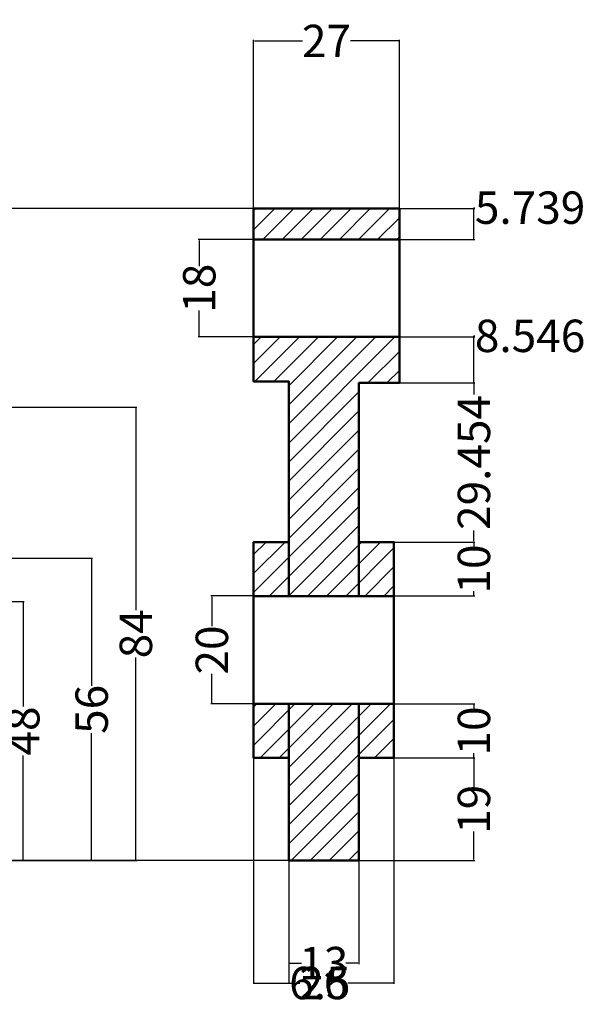
# Model space of a CAD drawing. Units: millimetres. Extents: x -1 to 307, y 9 to 193.
# Tile 2 of 2: x 203 to 307, y 11 to 193. Entities that reach past the tile are written whole.
import ezdxf

# ---------------------------------------------------------------- set-up
doc = ezdxf.new("R2010")
doc.units = ezdxf.units.MM
doc.header["$MEASUREMENT"] = 0
for name, color, linetype, lineweight in [('M-DIMS', 2, 'Continuous', 25), ('M-HATC', 8, 'Continuous', 18), ('M-OUTL', 7, 'Continuous', 50)]:
    doc.layers.add(name, color=color, linetype=linetype, lineweight=lineweight)
doc.styles.get("Standard").update_dxf_attribs({"font": 'arial.ttf'})
doc.dimstyles.get("Standard").update_dxf_attribs({"dimtxt": 6, "dimasz": 0.18, "dimexe": 0.18, "dimexo": 0.0625, "dimgap": 0.09, "dimtad": 0, "dimtoh": 1, "dimdec": 0, "dimzin": 0, "dimdsep": 46, "dimtxsty": 'Standard', "dimcen": 0.09, "dimadec": 0, "dimazin": 0, "dimtfac": 1, "dimtdec": 0, "dimtofl": 0, "dimtmove": 0, "dimatfit": 3, "dimfxl": 1, "dimtolj": 1, "dimtzin": 0, "dimarcsym": 0})

# ---------------------------------------------------------------- blocks, each defined once
blk = doc.blocks.new('*D1')
at = {"layer": 'Defpoints', "color": 0, "transparency": 16777216}
for p in [(252.51, 37.29), (265.51, 37.29), (265.51, 18.3)]:
    blk.add_point(p, dxfattribs=at)
at = {"layer": 'M-DIMS', "color": 0, "lineweight": -2, "transparency": 16777216}
for p, q in [((252.51, 37.23), (252.51, 18.12)), ((265.51, 37.23), (265.51, 18.12)), ((252.69, 18.3), (254.91, 18.3)), ((265.33, 18.3), (263.12, 18.3))]:
    blk.add_line(p, q, dxfattribs=at)
at = {"layer": 'M-DIMS', "color": 0, "transparency": 16777216}
for points in [[(252.69, 18.33), (252.69, 18.27), (252.51, 18.3)], [(265.33, 18.33), (265.33, 18.27), (265.51, 18.3)]]:
    blk.add_solid(points, dxfattribs=at)
at = {"layer": 'M-DIMS', "color": 0, "transparency": 16777216, "insert": (259.01, 18.3), "char_height": 6, "attachment_point": 5}
blk.add_mtext('\\A1;13', dxfattribs=at)
blk = doc.blocks.new('*D2')
at = {"layer": 'Defpoints', "color": 0, "transparency": 16777216}
for p in [(246.01, 86.29), (238.29, 66.29), (246.01, 66.29)]:
    blk.add_point(p, dxfattribs=at)
at = {"layer": 'M-DIMS', "color": 0, "lineweight": -2, "transparency": 16777216}
for p, q in [((245.95, 86.29), (238.11, 86.29)), ((238.29, 86.11), (238.29, 80.72)), ((238.29, 66.47), (238.29, 71.86)), ((245.95, 66.29), (238.11, 66.29))]:
    blk.add_line(p, q, dxfattribs=at)
at = {"layer": 'M-DIMS', "color": 0, "transparency": 16777216}
for points in [[(238.26, 86.11), (238.32, 86.11), (238.29, 86.29)], [(238.26, 66.47), (238.32, 66.47), (238.29, 66.29)]]:
    blk.add_solid(points, dxfattribs=at)
at = {"layer": 'M-DIMS', "color": 0, "transparency": 16777216, "insert": (238.29, 76.29), "char_height": 6, "attachment_point": 5, "rotation": 90}
blk.add_mtext('\\A1;20', dxfattribs=at)
blk = doc.blocks.new('*D3')
at = {"layer": 'Defpoints', "color": 0, "transparency": 16777216}
for p in [(246.01, 152.29), (235.95, 134.29), (246.01, 134.29)]:
    blk.add_point(p, dxfattribs=at)
at = {"layer": 'M-DIMS', "color": 0, "lineweight": -2, "transparency": 16777216}
for p, q in [((245.95, 152.29), (235.77, 152.29)), ((235.95, 152.11), (235.95, 147.4)), ((235.95, 134.47), (235.95, 139.18)), ((245.95, 134.29), (235.77, 134.29))]:
    blk.add_line(p, q, dxfattribs=at)
at = {"layer": 'M-DIMS', "color": 0, "transparency": 16777216}
for points in [[(235.92, 152.11), (235.98, 152.11), (235.95, 152.29)], [(235.92, 134.47), (235.98, 134.47), (235.95, 134.29)]]:
    blk.add_solid(points, dxfattribs=at)
at = {"layer": 'M-DIMS', "color": 0, "transparency": 16777216, "insert": (235.95, 143.29), "char_height": 6, "attachment_point": 5, "rotation": 90}
blk.add_mtext('\\A1;18', dxfattribs=at)
blk = doc.blocks.new('*D17')
at = {"layer": 'Defpoints', "color": 0, "transparency": 16777216}
for p in [(174.86, 85.29), (203.37, 85.29), (174.86, 37.29)]:
    blk.add_point(p, dxfattribs=at)
at = {"layer": 'M-DIMS', "color": 0, "lineweight": -2, "transparency": 16777216}
for p, q in [((174.93, 85.29), (203.55, 85.29)), ((203.37, 85.11), (203.37, 65.8)), ((203.37, 37.47), (203.37, 56.77)), ((174.93, 37.29), (203.55, 37.29))]:
    blk.add_line(p, q, dxfattribs=at)
at = {"layer": 'M-DIMS', "color": 0, "transparency": 16777216}
for points in [[(203.34, 85.11), (203.4, 85.11), (203.37, 85.29)], [(203.34, 37.47), (203.4, 37.47), (203.37, 37.29)]]:
    blk.add_solid(points, dxfattribs=at)
at = {"layer": 'M-DIMS', "color": 0, "transparency": 16777216, "insert": (203.37, 61.29), "char_height": 6, "attachment_point": 5, "rotation": 90}
blk.add_mtext('\\A1;48', dxfattribs=at)
blk = doc.blocks.new('*D18')
at = {"layer": 'Defpoints', "color": 0, "transparency": 16777216}
for p in [(190.86, 93.29), (216.03, 93.29), (174.86, 37.29)]:
    blk.add_point(p, dxfattribs=at)
at = {"layer": 'M-DIMS', "color": 0, "lineweight": -2, "transparency": 16777216}
for p, q in [((190.93, 93.29), (216.21, 93.29)), ((216.03, 93.11), (216.03, 69.67)), ((216.03, 37.47), (216.03, 60.9)), ((174.93, 37.29), (216.21, 37.29))]:
    blk.add_line(p, q, dxfattribs=at)
at = {"layer": 'M-DIMS', "color": 0, "transparency": 16777216}
for points in [[(216, 93.11), (216.06, 93.11), (216.03, 93.29)], [(216, 37.47), (216.06, 37.47), (216.03, 37.29)]]:
    blk.add_solid(points, dxfattribs=at)
at = {"layer": 'M-DIMS', "color": 0, "transparency": 16777216, "insert": (216.03, 65.29), "char_height": 6, "attachment_point": 5, "rotation": 90}
blk.add_mtext('\\A1;56', dxfattribs=at)
blk = doc.blocks.new('*D19')
at = {"layer": 'Defpoints', "color": 0, "transparency": 16777216}
for p in [(174.86, 121.29), (224.21, 121.29), (174.86, 37.29)]:
    blk.add_point(p, dxfattribs=at)
at = {"layer": 'M-DIMS', "color": 0, "lineweight": -2, "transparency": 16777216}
for p, q in [((174.93, 121.29), (224.39, 121.29)), ((224.21, 121.11), (224.21, 83.67)), ((224.21, 37.47), (224.21, 74.91)), ((174.93, 37.29), (224.39, 37.29))]:
    blk.add_line(p, q, dxfattribs=at)
at = {"layer": 'M-DIMS', "color": 0, "transparency": 16777216}
for points in [[(224.18, 121.11), (224.24, 121.11), (224.21, 121.29)], [(224.18, 37.47), (224.24, 37.47), (224.21, 37.29)]]:
    blk.add_solid(points, dxfattribs=at)
at = {"layer": 'M-DIMS', "color": 0, "transparency": 16777216, "insert": (224.21, 79.29), "char_height": 6, "attachment_point": 5, "rotation": 90}
blk.add_mtext('\\A1;84', dxfattribs=at)
blk = doc.blocks.new('*D29')
at = {"layer": 'Defpoints', "color": 0, "transparency": 16777216}
for p in [(3.06, 158.03), (246.01, 158.03), (252.51, 37.29)]:
    blk.add_point(p, dxfattribs=at)
at = {"layer": 'M-DIMS', "color": 0, "lineweight": -2, "transparency": 16777216}
for p, q in [((245.95, 158.03), (2.88, 158.03)), ((3.06, 157.85), (3.06, 109.91)), ((3.06, 37.47), (3.06, 85.41)), ((252.45, 37.29), (2.88, 37.29))]:
    blk.add_line(p, q, dxfattribs=at)
at = {"layer": 'M-DIMS', "color": 0, "transparency": 16777216}
for points in [[(3.03, 157.85), (3.09, 157.85), (3.06, 158.03)], [(3.03, 37.47), (3.09, 37.47), (3.06, 37.29)]]:
    blk.add_solid(points, dxfattribs=at)
at = {"layer": 'M-DIMS', "color": 0, "transparency": 16777216, "insert": (3.06, 97.66), "char_height": 6, "attachment_point": 5, "rotation": 90}
blk.add_mtext('\\A1;120.74', dxfattribs=at)
blk = doc.blocks.new('*D30')
at = {"layer": 'Defpoints', "color": 0, "transparency": 16777216}
for p in [(273.01, 189.09), (246.01, 158.03), (273.01, 158.03)]:
    blk.add_point(p, dxfattribs=at)
at = {"layer": 'M-DIMS', "color": 0, "lineweight": -2, "transparency": 16777216}
for p, q in [((246.01, 158.09), (246.01, 189.27)), ((246.19, 189.09), (255.07, 189.09)), ((272.83, 189.09), (263.95, 189.09)), ((273.01, 158.09), (273.01, 189.27))]:
    blk.add_line(p, q, dxfattribs=at)
at = {"layer": 'M-DIMS', "color": 0, "transparency": 16777216}
for points in [[(246.19, 189.12), (246.19, 189.06), (246.01, 189.09)], [(272.83, 189.12), (272.83, 189.06), (273.01, 189.09)]]:
    blk.add_solid(points, dxfattribs=at)
at = {"layer": 'M-DIMS', "color": 0, "transparency": 16777216, "insert": (259.51, 189.09), "char_height": 6, "attachment_point": 5}
blk.add_mtext('\\A1;27', dxfattribs=at)
blk = doc.blocks.new('*D31')
at = {"layer": 'Defpoints', "color": 0, "transparency": 16777216}
for p in [(246.01, 56.29), (272.01, 56.29), (272.01, 14.61)]:
    blk.add_point(p, dxfattribs=at)
at = {"layer": 'M-DIMS', "color": 0, "lineweight": -2, "transparency": 16777216}
for p, q in [((246.01, 56.23), (246.01, 14.43)), ((272.01, 56.23), (272.01, 14.43)), ((246.19, 14.61), (254.57, 14.61)), ((271.83, 14.61), (263.45, 14.61))]:
    blk.add_line(p, q, dxfattribs=at)
at = {"layer": 'M-DIMS', "color": 0, "transparency": 16777216}
for points in [[(246.19, 14.64), (246.19, 14.58), (246.01, 14.61)], [(271.83, 14.64), (271.83, 14.58), (272.01, 14.61)]]:
    blk.add_solid(points, dxfattribs=at)
at = {"layer": 'M-DIMS', "color": 0, "transparency": 16777216, "insert": (259.01, 14.61), "char_height": 6, "attachment_point": 5}
blk.add_mtext('\\A1;26', dxfattribs=at)
blk = doc.blocks.new('*D32')
at = {"layer": 'Defpoints', "color": 0, "transparency": 16777216}
for p in [(246.01, 56.29), (252.51, 56.29), (252.51, 14.61)]:
    blk.add_point(p, dxfattribs=at)
at = {"layer": 'M-DIMS', "color": 0, "lineweight": -2, "transparency": 16777216}
for p, q in [((246.01, 56.23), (246.01, 14.43)), ((252.51, 56.23), (252.51, 14.43)), ((246.19, 14.61), (252.33, 14.61)), ((252.51, 14.61), (252.69, 14.61))]:
    blk.add_line(p, q, dxfattribs=at)
at = {"layer": 'M-DIMS', "color": 0, "transparency": 16777216}
for points in [[(246.19, 14.64), (246.19, 14.58), (246.01, 14.61)], [(252.33, 14.64), (252.33, 14.58), (252.51, 14.61)]]:
    blk.add_solid(points, dxfattribs=at)
at = {"layer": 'M-DIMS', "color": 0, "transparency": 16777216, "insert": (258.28, 14.61), "char_height": 6, "attachment_point": 5}
blk.add_mtext('\\A1;6.5', dxfattribs=at)
blk = doc.blocks.new('*D33')
at = {"layer": 'Defpoints', "color": 0, "transparency": 16777216}
for p in [(273.01, 158.03), (286.81, 158.03), (273.01, 152.29)]:
    blk.add_point(p, dxfattribs=at)
at = {"layer": 'M-DIMS', "color": 0, "lineweight": -2, "transparency": 16777216}
for p, q in [((273.07, 158.03), (286.99, 158.03)), ((286.81, 158.03), (286.81, 158.21)), ((286.81, 158.21), (286.99, 158.21)), ((286.81, 152.47), (286.81, 157.85)), ((273.07, 152.29), (286.99, 152.29))]:
    blk.add_line(p, q, dxfattribs=at)
at = {"layer": 'M-DIMS', "color": 0, "transparency": 16777216}
for points in [[(286.78, 157.85), (286.84, 157.85), (286.81, 158.03)], [(286.78, 152.47), (286.84, 152.47), (286.81, 152.29)]]:
    blk.add_solid(points, dxfattribs=at)
at = {"layer": 'M-DIMS', "color": 0, "transparency": 16777216, "insert": (297.21, 158.21), "char_height": 6, "attachment_point": 5}
blk.add_mtext('\\A1;5.739', dxfattribs=at)
blk = doc.blocks.new('*D34')
at = {"layer": 'Defpoints', "color": 0, "transparency": 16777216}
for p in [(273.01, 134.29), (286.81, 134.29), (273.01, 125.74)]:
    blk.add_point(p, dxfattribs=at)
at = {"layer": 'M-DIMS', "color": 0, "lineweight": -2, "transparency": 16777216}
for p, q in [((273.07, 134.29), (286.99, 134.29)), ((286.81, 134.29), (286.81, 134.47)), ((286.81, 134.47), (286.99, 134.47)), ((286.81, 125.92), (286.81, 134.11)), ((273.07, 125.74), (286.99, 125.74))]:
    blk.add_line(p, q, dxfattribs=at)
at = {"layer": 'M-DIMS', "color": 0, "transparency": 16777216}
for points in [[(286.78, 134.11), (286.84, 134.11), (286.81, 134.29)], [(286.78, 125.92), (286.84, 125.92), (286.81, 125.74)]]:
    blk.add_solid(points, dxfattribs=at)
at = {"layer": 'M-DIMS', "color": 0, "transparency": 16777216, "insert": (297.21, 134.47), "char_height": 6, "attachment_point": 5}
blk.add_mtext('\\A1;8.546', dxfattribs=at)
blk = doc.blocks.new('*D35')
at = {"layer": 'Defpoints', "color": 0, "transparency": 16777216}
for p in [(273.01, 125.74), (286.81, 125.74), (272.01, 96.29)]:
    blk.add_point(p, dxfattribs=at)
at = {"layer": 'M-DIMS', "color": 0, "lineweight": -2, "transparency": 16777216}
for p, q in [((273.07, 125.74), (286.99, 125.74)), ((286.81, 125.56), (286.81, 123.6)), ((286.81, 96.47), (286.81, 98.43)), ((272.07, 96.29), (286.99, 96.29))]:
    blk.add_line(p, q, dxfattribs=at)
at = {"layer": 'M-DIMS', "color": 0, "transparency": 16777216}
for points in [[(286.78, 125.56), (286.84, 125.56), (286.81, 125.74)], [(286.78, 96.47), (286.84, 96.47), (286.81, 96.29)]]:
    blk.add_solid(points, dxfattribs=at)
at = {"layer": 'M-DIMS', "color": 0, "transparency": 16777216, "insert": (286.81, 111.02), "char_height": 6, "attachment_point": 5, "rotation": 90}
blk.add_mtext('\\A1;29.454', dxfattribs=at)
blk = doc.blocks.new('*D36')
at = {"layer": 'Defpoints', "color": 0, "transparency": 16777216}
for p in [(272.01, 96.29), (286.81, 96.29), (272.01, 86.29)]:
    blk.add_point(p, dxfattribs=at)
at = {"layer": 'M-DIMS', "color": 0, "lineweight": -2, "transparency": 16777216}
for p, q in [((272.07, 96.29), (286.99, 96.29)), ((286.81, 96.11), (286.81, 95.38)), ((272.07, 86.29), (286.99, 86.29)), ((286.81, 86.47), (286.81, 87.19))]:
    blk.add_line(p, q, dxfattribs=at)
at = {"layer": 'M-DIMS', "color": 0, "transparency": 16777216}
for points in [[(286.78, 96.11), (286.84, 96.11), (286.81, 96.29)], [(286.78, 86.47), (286.84, 86.47), (286.81, 86.29)]]:
    blk.add_solid(points, dxfattribs=at)
at = {"layer": 'M-DIMS', "color": 0, "transparency": 16777216, "insert": (286.81, 91.29), "char_height": 6, "attachment_point": 5, "rotation": 90}
blk.add_mtext('\\A1;10', dxfattribs=at)
blk = doc.blocks.new('*D37')
at = {"layer": 'Defpoints', "color": 0, "transparency": 16777216}
for p in [(272.01, 66.29), (286.81, 66.29), (272.01, 56.29)]:
    blk.add_point(p, dxfattribs=at)
at = {"layer": 'M-DIMS', "color": 0, "lineweight": -2, "transparency": 16777216}
for p, q in [((272.07, 66.29), (286.99, 66.29)), ((286.81, 66.11), (286.81, 65.38)), ((286.81, 56.47), (286.81, 57.19)), ((272.07, 56.29), (286.99, 56.29))]:
    blk.add_line(p, q, dxfattribs=at)
at = {"layer": 'M-DIMS', "color": 0, "transparency": 16777216}
for points in [[(286.78, 66.11), (286.84, 66.11), (286.81, 66.29)], [(286.78, 56.47), (286.84, 56.47), (286.81, 56.29)]]:
    blk.add_solid(points, dxfattribs=at)
at = {"layer": 'M-DIMS', "color": 0, "transparency": 16777216, "insert": (286.81, 61.29), "char_height": 6, "attachment_point": 5, "rotation": 90}
blk.add_mtext('\\A1;10', dxfattribs=at)
blk = doc.blocks.new('*D38')
at = {"layer": 'Defpoints', "color": 0, "transparency": 16777216}
for p in [(272.01, 56.29), (286.81, 56.29), (265.51, 37.29)]:
    blk.add_point(p, dxfattribs=at)
at = {"layer": 'M-DIMS', "color": 0, "lineweight": -2, "transparency": 16777216}
for p, q in [((272.07, 56.29), (286.99, 56.29)), ((286.81, 56.11), (286.81, 50.9)), ((286.81, 37.47), (286.81, 42.68)), ((265.57, 37.29), (286.99, 37.29))]:
    blk.add_line(p, q, dxfattribs=at)
at = {"layer": 'M-DIMS', "color": 0, "transparency": 16777216}
for points in [[(286.78, 56.11), (286.84, 56.11), (286.81, 56.29)], [(286.78, 37.47), (286.84, 37.47), (286.81, 37.29)]]:
    blk.add_solid(points, dxfattribs=at)
at = {"layer": 'M-DIMS', "color": 0, "transparency": 16777216, "insert": (286.81, 46.79), "char_height": 6, "attachment_point": 5, "rotation": 90}
blk.add_mtext('\\A1;19', dxfattribs=at)

msp = doc.modelspace()

# ---------------------------------------------------------------- hatches: boundary and pattern name
at = {"layer": 'M-HATC'}
h = msp.add_hatch(dxfattribs=at)
h.set_pattern_fill('ANSI31', color=256, scale=20)
h.paths.add_polyline_path([(273.0104, 158.0275), (246.0104, 158.0275), (246.0104, 152.2884), (273.0104, 152.2884)])
h = msp.add_hatch(dxfattribs=at)
h.set_pattern_fill('ANSI31', color=256, scale=20)
h.paths.add_polyline_path([(265.5104, 125.7421), (273.0104, 125.7421), (273.0104, 134.2884), (246.0104, 134.2884), (246.0104, 126.0275), (252.5104, 126.0275), (252.5104, 86.2884), (265.5104, 86.2884)])
h.paths.add_polyline_path([(252.5104, 96.2884), (246.0104, 96.2884), (246.0104, 86.2884), (252.5104, 86.2884)])
h.paths.add_polyline_path([(272.0104, 96.2884), (265.5104, 96.2884), (265.5104, 86.2884), (272.0104, 86.2884)], flags=17)
h.paths.add_polyline_path([(265.5104, 66.2884), (252.5104, 66.2884), (252.5104, 37.2884), (265.5104, 37.2884)])
h.paths.add_polyline_path([(252.5104, 66.2884), (246.0104, 66.2884), (246.0104, 56.2884), (252.5104, 56.2884)])
h.paths.add_polyline_path([(272.0104, 66.2884), (265.5104, 66.2884), (265.5104, 56.2884), (272.0104, 56.2884)])

# ---------------------------------------------------------------- linework, layer by layer
at = {"layer": 'M-OUTL'}
for p, q in [((246.0104, 152.2884), (273.0104, 152.2884)), ((246.0104, 134.2884), (273.0104, 134.2884)), ((246.0104, 86.2884), (272.0104, 86.2884))]:
    msp.add_line(p, q, dxfattribs=at)
for points in [[(252.5104, 86.2884), (252.5104, 126.0275), (246.0104, 126.0275), (246.0104, 158.0275), (273.0104, 158.0275), (273.0104, 125.7421)], [(265.5104, 86.2884), (265.5104, 125.7421), (273.0104, 125.7421)], [(252.5104, 56.2884), (246.0104, 56.2884), (246.0104, 96.2884), (252.5104, 96.2884)], [(265.5104, 56.2884), (265.5104, 56.2884), (272.0104, 56.2884), (272.0104, 96.2884), (265.5104, 96.2884)], [(246.0104, 66.2884), (252.5104, 66.2884), (272.0104, 66.2884)], [(265.5104, 66.2884), (265.5104, 37.2884), (252.5104, 37.2884), (252.5104, 66.2884)]]:
    msp.add_lwpolyline(points, dxfattribs=at)

# ---------------------------------------------------------------- dimensions: what is measured, and where the dimension line sits
at = {"layer": 'M-DIMS'}
for base, p1, p2, override, picture, middle in [((273.0104, 189.0884), (246.0104, 158.0275), (273.0104, 158.0275), {"dimdec": 0, "dimlfac": 1, "dimrnd": 0, "dimzin": 0, "dimdsep": 46, "dimlunit": 2}, '*D30', (259.5104, 189.0884)), ((272.0104, 14.6054), (246.0104, 56.2884), (272.0104, 56.2884), {"dimdec": 0, "dimlfac": 1, "dimrnd": 0, "dimzin": 0, "dimdsep": 46, "dimlunit": 2}, '*D31', (259.0104, 14.6054)), ((252.5104, 14.6054), (246.0104, 56.2884), (252.5104, 56.2884), {"dimdec": 1, "dimlfac": 1, "dimrnd": 0, "dimzin": 0, "dimdsep": 46, "dimlunit": 2}, '*D32', (258.2811, 14.6054)), ((265.5104, 18.2959), (252.5104, 37.2884), (265.5104, 37.2884), {"dimclrd": 0, "dimclre": 0, "dimclrt": 0}, '*D1', (259.0104, 18.2959))]:
    dim = msp.add_linear_dim(base=base, p1=p1, p2=p2, dimstyle='Standard', override=override, dxfattribs=at)
    dim.commit()
    dim.dimension.update_dxf_attribs({"geometry": picture, "text_midpoint": middle})
for base, p1, p2, override, picture, middle in [((286.8104, 158.0275), (273.0104, 152.2884), (273.0104, 158.0275), {"dimdec": 3, "dimlfac": 1, "dimrnd": 0, "dimzin": 0, "dimdsep": 46, "dimlunit": 2}, '*D33', (297.21, 158.2075)), ((3.0627, 158.0275), (252.5104, 37.2884), (246.0104, 158.0275), {"dimdec": 2, "dimlfac": 1, "dimrnd": 0, "dimzin": 0, "dimdsep": 46, "dimlunit": 2}, '*D29', (3.0627, 97.6579)), ((235.9456, 134.2884), (246.0104, 152.2884), (246.0104, 134.2884), {"dimclrd": 0, "dimclre": 0, "dimclrt": 0}, '*D3', (235.9456, 143.2884)), ((286.8104, 134.2884), (273.0104, 125.7421), (273.0104, 134.2884), {"dimdec": 3, "dimlfac": 1, "dimrnd": 0, "dimzin": 0, "dimdsep": 46, "dimlunit": 2}, '*D34', (297.2059, 134.4684)), ((286.8104, 125.7421), (272.0104, 96.2884), (273.0104, 125.7421), {"dimdec": 3, "dimlfac": 1, "dimrnd": 0, "dimzin": 0, "dimdsep": 46, "dimlunit": 2}, '*D35', (286.8104, 111.0152)), ((224.2119, 121.2884), (174.8627, 37.2884), (174.8627, 121.2884), {"dimclrd": 0, "dimclre": 0, "dimclrt": 0}, '*D19', (224.2119, 79.2884)), ((286.8104, 96.2884), (272.0104, 86.2884), (272.0104, 96.2884), {"dimdec": 0, "dimlfac": 1, "dimrnd": 0, "dimzin": 0, "dimdsep": 46, "dimlunit": 2}, '*D36', (286.8104, 91.2884)), ((216.0344, 93.2884), (174.8627, 37.2884), (190.8627, 93.2884), {"dimclrd": 0, "dimclre": 0, "dimclrt": 0}, '*D18', (216.0344, 65.2884)), ((238.2914, 66.2884), (246.0104, 86.2884), (246.0104, 66.2884), {"dimclrd": 0, "dimclre": 0, "dimclrt": 0}, '*D2', (238.2914, 76.2884)), ((203.3749, 85.2884), (174.8627, 37.2884), (174.8627, 85.2884), {"dimclrd": 0, "dimclre": 0, "dimclrt": 0}, '*D17', (203.3749, 61.2884)), ((286.8104, 66.2884), (272.0104, 56.2884), (272.0104, 66.2884), {"dimdec": 0, "dimlfac": 1, "dimrnd": 0, "dimzin": 0, "dimdsep": 46, "dimlunit": 2}, '*D37', (286.8104, 61.2884)), ((286.8104, 56.2884), (265.5104, 37.2884), (272.0104, 56.2884), {"dimdec": 0, "dimlfac": 1, "dimrnd": 0, "dimzin": 0, "dimdsep": 46, "dimlunit": 2}, '*D38', (286.8104, 46.7884))]:
    dim = msp.add_linear_dim(base=base, p1=p1, p2=p2, angle=90, dimstyle='Standard', override=override, dxfattribs=at)
    dim.commit()
    dim.dimension.update_dxf_attribs({"geometry": picture, "text_midpoint": middle})

doc.saveas('drawing.dxf')
